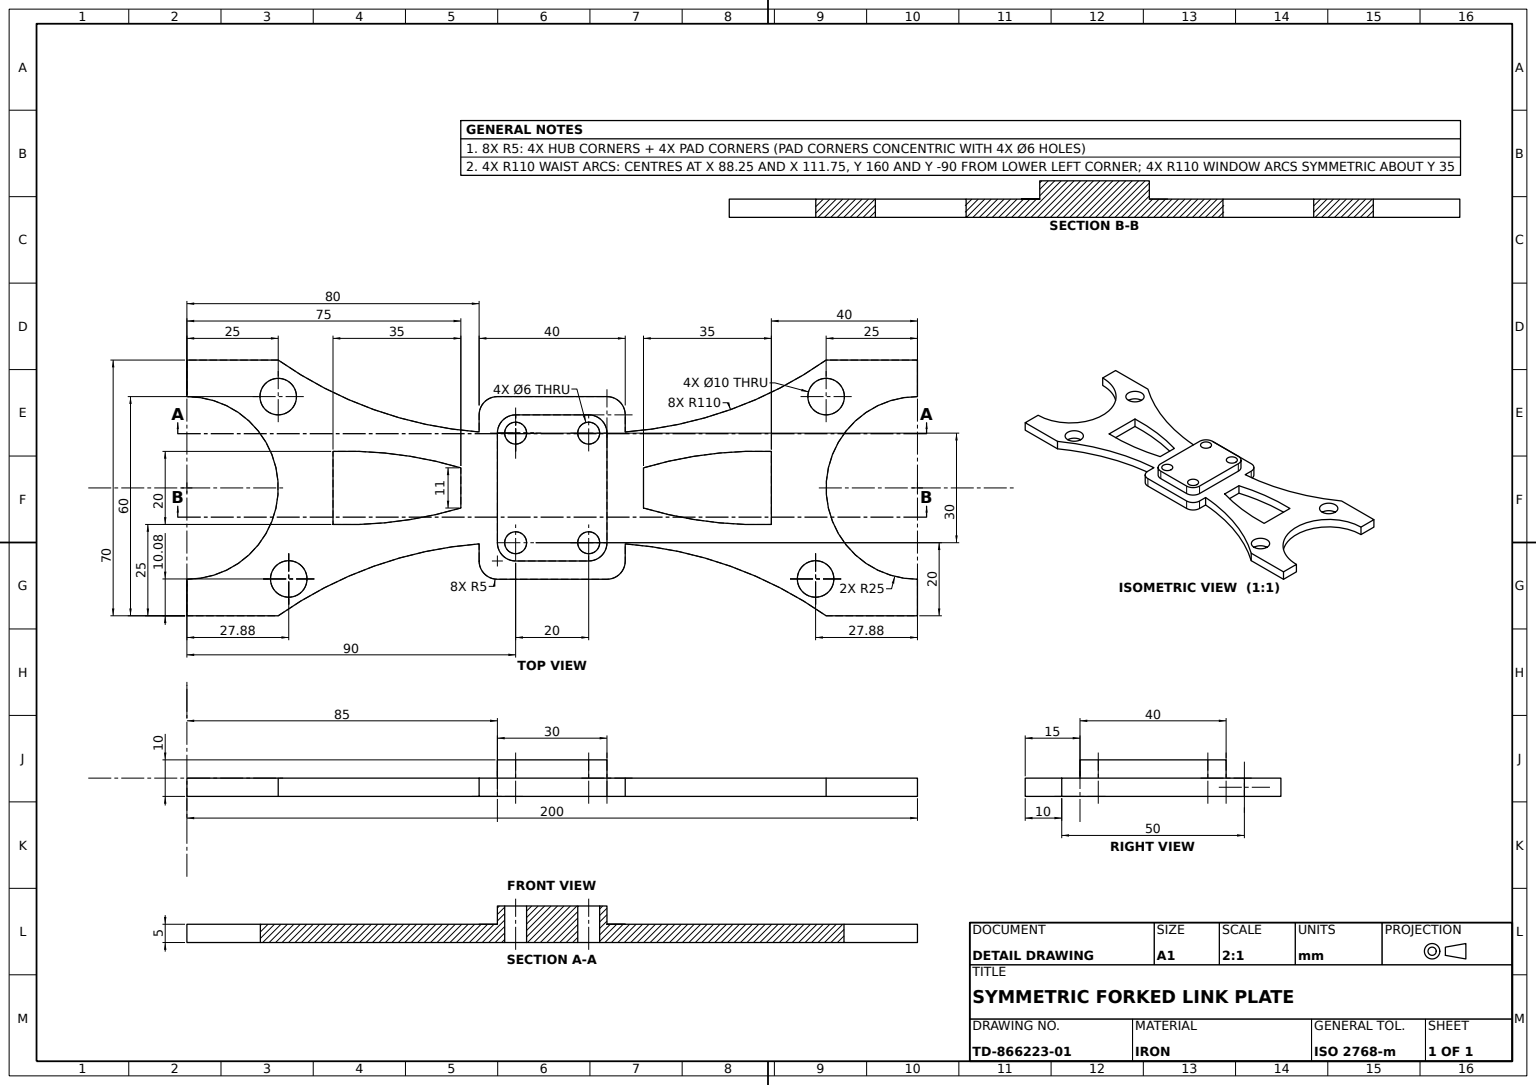
CATIA V5 part; units mm, degrees
sketch "Sketch1" plane through (0, 0, 0) normal (0, 0, 1) x (1, 0, 0)
  line L0 (20, 25) -> (20, 15.3095)
  line L1 (20, -25) -> (-20, -25)
  line L2 (-20, -25) -> (-20, -15.3095)
  line L3 (-20, 25) -> (20, 25)
  point P0 (20, 25)
  point P1 (20, -25)
  line L4 (-99.5847, 0) -> (118.3951, 0) construction
  point P2 (-99.5847, 0)
  arc A0 (100, 25) -> (100, -25) centre (100, 0) ccw
  point P3 (100, 0)
  arc A1 (20, 15.3095) -> (75, 35) centre (11.7544, 125) ccw
  line L5 (15, 20) -> (15, -20) construction
  line L6 (15, -20) -> (-15, -20) construction
  line L7 (-15, -20) -> (-15, 20) construction
  line L8 (-15, 20) -> (15, 20) construction
  arc A2 (-10, 20) -> (-15, 15) centre (-10, 15) ccw construction
  point P4 (-10, 20)
  point P5 (-15, 15)
  arc A3 (-10, -20) -> (-15, -15) centre (-10, -15) cw construction
  point P6 (-10, -20)
  point P7 (-15, -15)
  point P8 (15, 15)
  point P9 (10, 20)
  arc A4 (10, 20) -> (15, 15) centre (10, 15) cw construction
  point P10 (15, -15)
  point P11 (10, -20)
  arc A5 (10, -20) -> (15, -15) centre (10, -15) ccw construction
  circle A6 centre (10, 15) radius 3 construction
  circle A7 centre (75, 25) radius 5
  point P12 (75, 25)
  circle A8 centre (72.1162, -24.9168) radius 5
  point P13 (72.1162, -24.9168)
  line L9 (100, 25) -> (100, 35)
  point P14 (100, 25)
  point P15 (100, 35)
  line L10 (100, 25) -> (75, 25) construction
  line L11 (100, -25) -> (100, -35)
  point P16 (100, -25)
  point P17 (100, -35)
  line L12 (100, -35) -> (75, -35)
  point P18 (75, -35)
  line L13 (100, 35) -> (75, 35)
  point P19 (75, 35)
  point P20 (20, 15.3095)
  point P21 (75, -35)
  point P22 (20, -15.3095)
  arc A9 (20, -15.3095) -> (75, -35) centre (11.7544, -125) cw
  line L14 (60, -10) -> (60, 10)
  point P23 (60, 0)
  point P24 (60, -10)
  point P25 (60, 10)
  line L15 (25, -5.5) -> (25, 5.5)
  point P26 (25, 0)
  point P27 (25, -5.5)
  point P28 (25, 5.5)
  arc A10 (60, -10) -> (25, -5.5) centre (56.3458, 99.9393) cw
  point P29 (25, 5.5)
  point P30 (60, 10)
  arc A11 (60, 10) -> (25, 5.5) centre (56.3458, -99.9393) ccw
  point P31 (-75, -35)
  point P32 (-20, -15.3095)
  arc A12 (-20, -15.3095) -> (-75, -35) centre (-11.7544, -125) ccw
  point P33 (-25, -5.5)
  point P34 (-60, -10)
  arc A13 (-60, -10) -> (-25, -5.5) centre (-56.3458, 99.9393) ccw
  point P35 (-60, 10)
  line L16 (-60, -10) -> (-60, 10)
  point P36 (-25, 5.5)
  point P37 (-60, 10)
  arc A14 (-60, 10) -> (-25, 5.5) centre (-56.3458, -99.9393) cw
  point P38 (-75, 35)
  point P39 (-20, 15.3095)
  arc A15 (-20, 15.3095) -> (-75, 35) centre (-11.7544, 125) cw
  point P40 (-100, 35)
  line L17 (-100, 35) -> (-75, 35)
  point P41 (-100, -25)
  point P42 (-100, 25)
  arc A16 (-100, 25) -> (-100, -25) centre (-100, 0) cw
  circle A17 centre (-72.1162, -24.9168) radius 5
  circle A18 centre (-75, 25) radius 5
  point P43 (-75, -35)
  point P44 (-100, -35)
  line L18 (-100, -35) -> (-75, -35)
  line L19 (-100, -25) -> (-100, -35)
  point P45 (-25, 5.5)
  point P46 (-25, -5.5)
  line L20 (-25, -5.5) -> (-25, 5.5)
  point P47 (-100, 35)
  point P48 (-100, 25)
  line L21 (-100, 25) -> (-100, 35)
  line L22 (20, -15.3095) -> (20, -25)
  line L23 (-20, 15.3095) -> (-20, 25)
  dimension "length L1" = 40
  dimension "radius A0" = 25
  dimension "radius A1" = 110
  dimension "length L6" = 30
  dimension "length L5" = 40
  dimension "radius A2" = 5
  dimension "radius A3" = 5
  dimension "radius A6" = 3
  dimension "radius A7" = 5
  dimension "radius A8" = 5
  dimension "distance P12 P13" = 50
  dimension "distance P12 L4" = 25
  dimension "distance y axis A8" = 67.1162
  dimension "length L9" = 10
  dimension "length L10" = 25
  dimension "length L11" = 10
  dimension "length L13" = 25
  dimension "length L12" = 25
  dimension "length L14" = 20
  dimension "length L15" = 11
  dimension "distance L14 L15" = 35
  dimension "radius A10" = 110
  dimension "distance P0 P1" = 50
  dimension "distance L14 L9" = 40
  dimension "distance A9 A8" = 1.8768
  dimension "distance A1 A7" = 3.3216
  constraint vertical L0 y-axis
  constraint vertical L2 y-axis
  constraint vertical L5 y-axis
  constraint vertical L7 y-axis
  constraint vertical L9 y-axis
  constraint vertical L11 y-axis
  constraint vertical L14 y-axis
  constraint vertical L15 y-axis
  constraint vertical L22 y-axis
  constraint vertical L23 y-axis
  constraint horizontal L1 x-axis
  constraint horizontal L3 x-axis
  constraint horizontal L4 x-axis
  constraint horizontal L6 x-axis
  constraint horizontal L8 x-axis
  constraint horizontal L12 x-axis
  constraint horizontal L13 x-axis
  constraint equidistance L0 L2 origin
  constraint equidistance L1 L3 origin
  constraint equidistance L5 L7 origin
  constraint equidistance L6 L8 origin
  constraint coincidence P2 x-axis
  constraint coincidence P3 L4
  constraint coincidence L8 P4
  constraint coincidence L7 P5
  constraint coincidence L6 P6
  constraint coincidence L7 P7
  constraint coincidence P14 L3
  constraint coincidence P16 L9
  constraint coincidence P23 L4
  constraint coincidence P26 L4
  constraint coincidence L0 L22
  constraint coincidence L2 L23
  constraint coincidence P25 P30
  constraint coincidence P28 P29
  constraint coincidence P33 P46
  constraint coincidence P35 P37
  constraint coincidence P36 P45
  constraint coincidence L9 L11
  constraint tangency A2 L8
  constraint tangency A2 L7
  constraint tangency A3 L6
  constraint tangency A3 L7
  constraint symmetry P5 P8 y-axis
  constraint symmetry P4 P9 y-axis
  constraint symmetry A2 A4 y-axis
  constraint symmetry P7 P10 y-axis
  constraint symmetry P6 P11 y-axis
  constraint symmetry A3 A5 y-axis
  constraint symmetry P19 P21 L4
  constraint symmetry P20 P22 L4
  constraint symmetry A1 A9 L4
  constraint symmetry P27 P29 L4
  constraint symmetry P24 P30 L4
  constraint symmetry A10 A11 L4
  constraint symmetry P21 P31 y-axis
  constraint symmetry P22 P32 y-axis
  constraint symmetry A9 A12 y-axis
  constraint symmetry P27 P33 y-axis
  constraint symmetry P24 P34 y-axis
  constraint symmetry A10 A13 y-axis
  constraint symmetry P25 P35 y-axis
  constraint symmetry L14 L16 y-axis
  constraint symmetry P29 P36 y-axis
  constraint symmetry P30 P37 y-axis
  constraint symmetry A11 A14 y-axis
  constraint symmetry P19 P38 y-axis
  constraint symmetry P20 P39 y-axis
  constraint symmetry A1 A15 y-axis
  constraint symmetry P15 P40 y-axis
  constraint symmetry L13 L17 y-axis
  constraint symmetry P16 P41 y-axis
  constraint symmetry P14 P42 y-axis
  constraint symmetry A0 A16 y-axis
  constraint symmetry A8 A17 y-axis
  constraint symmetry A7 A18 y-axis
  constraint symmetry P18 P43 y-axis
  constraint symmetry P17 P44 y-axis
  constraint symmetry L12 L18 y-axis
  constraint symmetry L11 L19 y-axis
  constraint symmetry P28 P45 y-axis
  constraint symmetry P27 P46 y-axis
  constraint symmetry L15 L20 y-axis
  constraint symmetry P15 P47 y-axis
  constraint symmetry P14 P48 y-axis
  constraint symmetry L9 L21 y-axis
  constraint midpoint L14 P23
  constraint midpoint L15 P26
extrude "Pad1" add sketch "Sketch1" against normal blind 5
sketch "Sketch2" plane through (0, 0, 0) normal (0, 0, 1) x (1, 0, 0)
  line L0 (15, 20) -> (15, -20)
  line L1 (15, -20) -> (-15, -20)
  line L2 (-15, -20) -> (-15, 20)
  line L3 (-15, 20) -> (15, 20)
  point P0 (10, 15)
  circle A0 centre (10, 15) radius 3
  circle A1 centre (10, -15) radius 3
  point P1 (10, -15)
  circle A2 centre (-10, -15) radius 3
  point P2 (-10, -15)
  circle A3 centre (-10, 15.0002) radius 3
  point P3 (-10, 15.0002)
  dimension "length L1" = 30
  dimension "length L0" = 40
  dimension "radius A0" = 3
  dimension "distance P0 L3" = 5
  dimension "distance P0 L0" = 5
  dimension "radius A1" = 3
  dimension "radius A2" = 3
  dimension "radius A3" = 3
  dimension "distance P3 L2" = 5
  dimension "distance P3 L3" = 4.9998
  dimension "distance P1 L1" = 5
  dimension "distance P1 L0" = 5
  dimension "distance P2 L1" = 5
  dimension "distance P2 L2" = 5
  constraint vertical L0 y-axis
  constraint vertical L2 y-axis
  constraint horizontal L1 x-axis
  constraint horizontal L3 x-axis
  constraint equidistance L0 L2 origin
  constraint equidistance L1 L3 origin
extrude "Pad2" add sketch "Sketch2" along normal blind 5
sketch "Sketch3" plane through (0, 0, 0) normal (0, 0, 1) x (1, 0, 0)
  circle A0 centre (10, 15) radius 3
  circle A1 centre (10, -15) radius 3
  circle A2 centre (-10, 15.0002) radius 3
  circle A3 centre (-10, -15) radius 3
extrude "Pocket1" cut sketch "Sketch3" against normal blind 20
fillet "Fillet1" radius 5 8 edges at (15, 20, 2.5) (-15, 20, 2.5) (15, -20, 2.5) (20, -25, -2.5) (20, 25, -2.5) (-20, 25, -2.5) (-15, -20, 2.5) (-20, -25, -2.5)
properties material "Iron"
